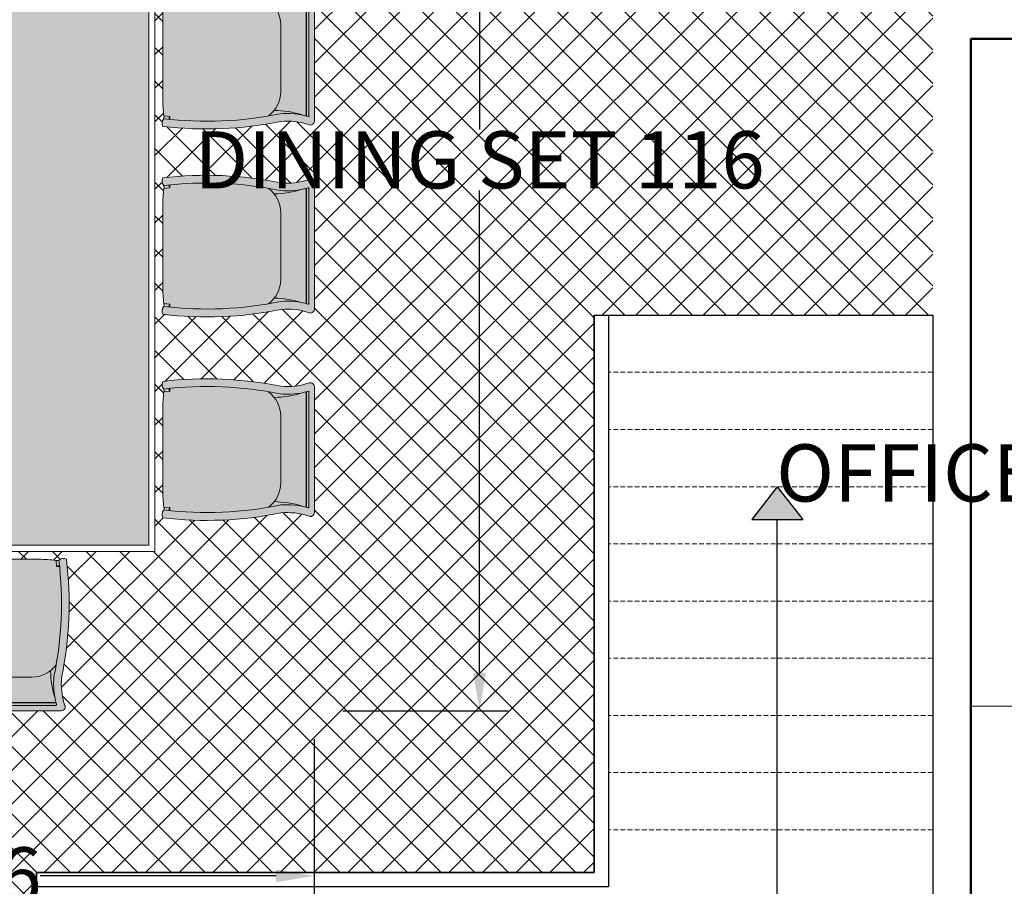
# Model space of a CAD drawing. Units: inches. Extents: x -466983 to 1020, y 324 to 318697.
# Tile 30 of 97: x 714 to 817, y 736 to 827. Entities that reach past the tile are written whole.
import ezdxf

# ---------------------------------------------------------------- set-up
doc = ezdxf.new("R2010")
doc.units = ezdxf.units.IN
doc.header["$MEASUREMENT"] = 0
doc.linetypes.add('DASHED', pattern=[0.75, 0.5, -0.25])
for name, color, linetype, lineweight in [('A-ANNO-DIMS', 2, 'Continuous', 18), ('A-FLOR-PATT', 252, 'Continuous', 13), ('A-FLOR-STRS', 30, 'Continuous', 25), ('A-FLOR-STRS-OVHD', 30, 'DASHED', 18), ('A-FURN', 8, 'Continuous', 18), ('A-WALL', 7, 'Continuous', 50)]:
    doc.layers.add(name, color=color, linetype=linetype, lineweight=lineweight)
doc.styles.get("Standard").update_dxf_attribs({"font": 'arial.ttf'})
doc.dimstyles.get("Standard").update_dxf_attribs({"dimtxt": 6, "dimasz": 4, "dimexe": 3, "dimexo": 3, "dimgap": 0.09, "dimtad": 0, "dimtih": 1, "dimtoh": 1, "dimdec": 1, "dimzin": 0, "dimdsep": 46, "dimlunit": 3, "dimtxsty": 'Standard', "dimcen": 0.09, "dimadec": 0, "dimazin": 0, "dimtfac": 1, "dimtdec": 1, "dimtofl": 0, "dimtmove": 0, "dimatfit": 3, "dimfxl": 1, "dimtolj": 1, "dimtzin": 0, "dimarcsym": 0})

# ---------------------------------------------------------------- blocks, each defined once
blk = doc.blocks.new('A$C51F1')
h = blk.add_hatch(color=256)
h.dxf.hatch_style = 1
h.paths.add_polyline_path([(0.4279, 0.4929), (0.026, 0.4929, 0.585109), (0.0153, 0.4737, -0.102523), (0.0249, 0.3863, 0.080461), (0.0093, 0.0091, 0.3023), (0.0338, 0.012, -0.012942), (0.0343, 0.0123, -0.080591), (0.05, 0.3835, 0.086627), (0.0435, 0.4661, -0.308377), (0.0433, 0.4665, -0.237278), (0.0433, 0.4671, 0.005839), (0.0418, 0.4726, -0.471786), (0.0436, 0.4758), (0.2273, 0.4758), (0.4111, 0.4758, -0.471786), (0.4129, 0.4726, 0.005839), (0.4114, 0.4671, -0.293853), (0.4112, 0.4664, 0.08699), (0.4047, 0.3835, -0.080655), (0.4203, 0.012, 0.301773), (0.4447, 0.0091, 0.080461), (0.4291, 0.3863, -0.102523), (0.4387, 0.4737, 0.587111)])
h.paths.add_polyline_path([(0.4107, 0.4676), (0.2273, 0.4676), (0.0439, 0.4676, 0.311255), (0.0433, 0.4671, -0.000568), (0.0434, 0.4666, -0.365297), (0.0439, 0.4668), (0.2273, 0.4668), (0.4107, 0.4668, -0.365297), (0.4113, 0.4666, -0.000568), (0.4114, 0.4671, 0.311255)], flags=17)
h = blk.add_hatch(color=256)
h.dxf.hatch_style = 1
h.paths.add_polyline_path([(0.4117, 0.3464, 0.23459), (0.3341, 0.3858), (0.2273, 0.3858), (0.1205, 0.3858, 0.165743), (0.061, 0.3649, 0.071703), (0.0463, 0.4542, -0.071168), (0.0502, 0.3861, 0.080361), (0.0343, 0.0123, -0.184513), (0.0429, 0.0127, 0.028193), (0.097, 0.0091), (0.227, 0.0091), (0.3571, 0.0091, 0.028193), (0.4111, 0.0127, -0.198751), (0.4203, 0.012, 0.072468)])
h.paths.add_polyline_path([(0.4084, 0.4542, -0.01323), (0.4113, 0.4666, 0.365297), (0.4107, 0.4668, 0.310553), (0.4107, 0.4676), (0.0439, 0.4676, 0.311255), (0.0433, 0.4671, -0.013798), (0.0463, 0.4542, -0.071703), (0.061, 0.3649, -0.165743), (0.1205, 0.3858), (0.2273, 0.3858), (0.3341, 0.3858, -0.165743), (0.3937, 0.3649, -0.071703)])
h.paths.add_polyline_path([(0.4047, 0.3835, -0.073923), (0.4084, 0.4542, 0.071703), (0.3937, 0.3649, -0.06627), (0.4117, 0.3464, 0.008137)], flags=17)
h.paths.add_polyline_path([(0.413, 0.473, 0.415817), (0.4111, 0.4758), (0.0436, 0.4758, 0.415817), (0.0416, 0.473, -0.006308), (0.0433, 0.4671, -0.311255), (0.0439, 0.4676), (0.4107, 0.4676, -0.336555), (0.4114, 0.4671, -0.006308)])
h = blk.add_hatch(color=256)
h.dxf.hatch_style = 1
h.paths.add_polyline_path([(0.4084, 0.4542, -0.01323), (0.4113, 0.4666, 0.365297), (0.4107, 0.4668), (0.2273, 0.4668), (0.0436, 0.4668, 0.193526), (0.0434, 0.4666, -0.01323), (0.0463, 0.4542, -0.071703), (0.061, 0.3649, -0.165743), (0.1205, 0.3858), (0.2273, 0.3858), (0.3341, 0.3858, -0.165743), (0.3937, 0.3649, -0.071703)])
at = {"color": 0}
for p, q in [((0.0436, 0.4758), (0.4111, 0.4758)), ((0.0439, 0.4676), (0.4107, 0.4676)), ((0.2273, 0.4668), (0.0439, 0.4668)), ((0.2273, 0.4668), (0.4107, 0.4668)), ((0.2273, 0.3858), (0.1205, 0.3858)), ((0.2273, 0.3858), (0.3341, 0.3858)), ((0.0417, 0.0321), (0.0321, 0.0321)), ((0.0417, 0.0321), (0.0326, 0.0278)), ((0.0435, 0.0127), (0.0417, 0.0321)), ((0.4112, 0.0127), (0.4129, 0.0321)), ((0.4129, 0.0321), (0.4225, 0.0321)), ((0.4129, 0.0321), (0.4221, 0.0278))]:
    blk.add_line(p, q, dxfattribs=at)
blk.add_lwpolyline([(0.4387, 0.4737, 0.102523), (0.4291, 0.3863, -0.080461), (0.4447, 0.0091, -0.3023), (0.4203, 0.012, 0.197932), (0.4111, 0.0127, -0.028193), (0.3571, 0.0091), (0.227, 0.0091), (0.097, 0.0091, -0.028193), (0.0429, 0.0127, 0.197932), (0.0338, 0.012, -0.3023), (0.0093, 0.0091, -0.080461), (0.0249, 0.3863, 0.102523), (0.0153, 0.4737, -0.587111), (0.0261, 0.4929), (0.4279, 0.4929, -0.587111)], format="xyb", close=True, dxfattribs=at)
for centre, radius, start, end in [((0.044, 0.4735), 0.00242, 100.345, 201.3742), ((-0.1898, 0.4063), 0.2409, 355.1793, 16.07), ((0.6445, 0.4063), 0.2409, 164.0374, 185.4487), ((0.4106, 0.4735), 0.00242, 338.6258, 79.655), ((0.0439, 0.4669), 0.000725, 87.3762, 197.5208), ((0.0438, 0.4664), 0.000433, 71.7715, 189.2202), ((-0.2563, 0.3584), 0.3173, 1.1591, 17.5641), ((0.7109, 0.3584), 0.3173, 162.4359, 178.8409), ((0.4107, 0.4669), 0.000725, 342.4792, 92.6238), ((0.4109, 0.4664), 0.000433, 350.7798, 108.2285), ((1.1976, 0.1501), 1.1714, 168.378, 186.769), ((0.1214, 0.2879), 0.0978, 90.5164, 143.1927), ((0.3332, 0.2879), 0.0978, 36.8073, 89.4836), ((-0.7314, 0.1497), 1.1599, 353.1854, 11.6291), ((0.0397, 0.0013), 0.012, 71.7536, 116.5375), ((0.4149, 0.0013), 0.012, 63.4625, 108.2464)]:
    blk.add_arc(centre, radius, start, end, dxfattribs=at)
blk = doc.blocks.new('Dining Table 1')
h = blk.add_hatch(color=256)
h.dxf.hatch_style = 1
h.set_gradient(color1=(0, 107, 0), color2=(254, 234, 185), name='INVSPHERICAL')
h.paths.add_polyline_path([(1939.98, 1142.68), (1908.44, 1142.68), (1908.44, 1061.84), (1939.98, 1061.84)])
at = {"ltscale": 0.5}
for points in [[(1907.78, 1143.33), (1907.78, 1061.19), (1940.64, 1061.19), (1940.64, 1143.33)], [(1908.44, 1142.68), (1908.44, 1061.84), (1939.98, 1061.84), (1939.98, 1142.68)]]:
    blk.add_lwpolyline(points, close=True, dxfattribs=at)
at = {"ltscale": 0.5, "xscale": 32.85880592291654, "yscale": 32.85880592291654, "zscale": 32.85880592291654}
blk.add_blockref('A$C51F1', (1916.75, 1143.86), dxfattribs=at)
at = {"ltscale": 0.5, "yscale": 32.85880592291654, "zscale": 32.85880592291654}
for p, xscale, rotation in [((1907.26, 1140.11), -32.85880592291654, 90), ((1941.16, 1140.11), 32.85880592291654, 270), ((1907.26, 1120.4), -32.85880592291654, 90), ((1941.16, 1120.4), 32.85880592291654, 270), ((1907.26, 1085.76), 32.85880592291654, 89.99999999999999), ((1941.16, 1085.76), -32.85880592291654, 270), ((1907.26, 1064.41), 32.85880592291654, 89.99999999999999), ((1941.16, 1064.41), -32.85880592291654, 270), ((1916.75, 1060.66), -32.85880592291654, 180)]:
    blk.add_blockref('A$C51F1', p, dxfattribs=dict(at, xscale=xscale, rotation=rotation))
blk = doc.blocks.new('*D99')
at = {"layer": 'A-ANNO-DIMS', "color": 0, "lineweight": -2, "transparency": 16777216}
for p, q in [((833.84, 822.68), (820.85, 822.68)), ((823.85, 818.68), (823.85, 782.57)), ((823.85, 740.08), (823.85, 776.18)), ((833.84, 736.08), (820.85, 736.08))]:
    blk.add_line(p, q, dxfattribs=at)
at = {"layer": 'A-ANNO-DIMS', "color": 0, "transparency": 16777216}
for points in [[(823.18, 818.68), (824.52, 818.68), (823.85, 822.68)], [(823.18, 740.08), (824.52, 740.08), (823.85, 736.08)]]:
    blk.add_solid(points, dxfattribs=at)
at = {"layer": 'Defpoints', "color": 0, "transparency": 16777216}
for p in [(823.85, 822.68), (836.84, 822.68), (836.84, 736.08)]:
    blk.add_point(p, dxfattribs=at)
at = {"layer": 'A-ANNO-DIMS', "color": 0, "transparency": 16777216, "insert": (823.85, 779.38), "char_height": 6, "attachment_point": 5}
blk.add_mtext('\\A1;OFFICE DESK 87', dxfattribs=at)
blk = doc.blocks.new('*D111')
at = {"layer": 'A-ANNO-DIMS', "color": 0, "lineweight": -2, "transparency": 16777216}
for p, q in [((747.94, 870.02), (765.28, 870.02)), ((762.28, 866.02), (762.28, 815.42)), ((762.28, 758.43), (762.28, 809.03)), ((747.94, 754.43), (765.28, 754.43))]:
    blk.add_line(p, q, dxfattribs=at)
at = {"layer": 'A-ANNO-DIMS', "color": 0, "transparency": 16777216}
for points in [[(761.61, 866.02), (762.95, 866.02), (762.28, 870.02)], [(761.61, 758.43), (762.95, 758.43), (762.28, 754.43)]]:
    blk.add_solid(points, dxfattribs=at)
at = {"layer": 'Defpoints', "color": 0, "transparency": 16777216}
for p in [(744.94, 870.02), (762.28, 870.02), (744.94, 754.43)]:
    blk.add_point(p, dxfattribs=at)
at = {"layer": 'A-ANNO-DIMS', "color": 0, "transparency": 16777216, "insert": (762.28, 812.23), "char_height": 6, "attachment_point": 5}
blk.add_mtext('\\A1;DINING SET 116', dxfattribs=at)
blk = doc.blocks.new('*D112')
at = {"layer": 'A-ANNO-DIMS', "color": 0, "lineweight": -2, "transparency": 16777216}
for p, q in [((678.65, 751.43), (678.65, 734.1)), ((744.94, 751.43), (744.94, 734.1)), ((682.65, 737.1), (707.39, 737.1)), ((740.94, 737.1), (716.2, 737.1))]:
    blk.add_line(p, q, dxfattribs=at)
at = {"layer": 'A-ANNO-DIMS', "color": 0, "transparency": 16777216}
for points in [[(682.65, 737.76), (682.65, 736.43), (678.65, 737.1)], [(740.94, 737.76), (740.94, 736.43), (744.94, 737.1)]]:
    blk.add_solid(points, dxfattribs=at)
at = {"layer": 'Defpoints', "color": 0, "transparency": 16777216}
for p in [(678.65, 754.43), (744.94, 754.43), (744.94, 737.1)]:
    blk.add_point(p, dxfattribs=at)
at = {"layer": 'A-ANNO-DIMS', "color": 0, "transparency": 16777216, "insert": (711.79, 737.1), "char_height": 6, "attachment_point": 5}
blk.add_mtext('\\A1;66', dxfattribs=at)

msp = doc.modelspace()

# ---------------------------------------------------------------- hatches: boundary and pattern name
at = {"layer": 'A-FLOR-PATT', "transparency": 33554572}
h = msp.add_hatch(dxfattribs=at)
h.set_pattern_fill('ANSI37', color=256, scale=30)
h.set_pattern_definition([(45, (-1212.4137, -290.035), (-2.6516504, 2.6516504), []), (135, (-1212.4137, -290.035), (-2.6516504, -2.6516504), [])])
h.paths.add_polyline_path([(901.81, 1075.94), (900.61, 1075.94), (900.61, 1065.39), (899.39, 1065.39), (898.09, 1065.39), (892.84, 1058.71, -0.258377), (892.19, 1058.35), (879.98, 1058.35, -0.20177), (879.44, 1058.58), (874.08, 1065.39), (872.78, 1065.39), (871.56, 1065.39), (871.56, 1075.94), (813.81, 1075.94), (813.81, 1044.79), (832.39, 1044.79, -0.394795), (848.66, 1028.54), (848.66, 1009.94), (901.81, 1009.94), (901.81, 1015.94), (901.31, 1015.94), (871.31, 1015.94), (871.31, 1017.25), (871.33, 1017.25, -0.401453), (901.31, 1045.94), (901.81, 1045.94)])
edge = h.paths.add_edge_path(flags=16)
edge.add_line((847.77, 1068.95), (847.77, 1073.71))
edge.add_arc((849.23, 1073.71), 1.45, 90, 180, ccw=False)
edge.add_line((849.23, 1075.16), (864.49, 1075.16))
edge.add_arc((864.49, 1073.71), 1.45, 0, 90, ccw=False)
edge.add_line((865.95, 1073.71), (865.95, 1069))
edge.add_arc((832.64, 1068.98), 33.3, -20.6123, 0.0472, ccw=False)
edge.add_ellipse((856.86, 1058.48), major_axis=(0, 10.21), ratio=0.685919, start_angle=100.0088, end_angle=259.9912, ccw=False)
edge.add_arc((881.07, 1068.98), 33.3, 180.0472, 200.6123, ccw=False)
h.paths.add_polyline_path([(853.15, 1066.48), (853.15, 1066.45), (853.15, 1066.45, 0.433107), (852.92, 1066.68), (852.92, 1066.45), (853.15, 1066.45), (853.15, 1066.48), (853.09, 1066.61, 0.697939), (852.7, 1066.45), (852.7, 1066.45), (852.7, 1066.48), (852.92, 1067), (852.92, 1066.68, -0.396254)], flags=0)
h.paths.add_polyline_path([(861.02, 1066.48), (861.02, 1066.45), (861.02, 1066.45, 0.416404), (860.8, 1066.68), (860.8, 1066.45), (861.02, 1066.45), (861.02, 1066.48), (860.97, 1066.61, 0.713344), (860.57, 1066.45), (860.57, 1066.45), (860.57, 1066.48), (860.8, 1067), (860.8, 1066.68, -0.379973)], flags=0)
edge = h.paths.add_edge_path(flags=0)
edge.add_spline(control_points=[(861.13, 1065.79), (861.47, 1065.25), (861.61, 1065.02), (861.98, 1064.37), (862.19, 1063.94), (862.56, 1063.04), (862.72, 1062.56), (862.99, 1061.58), (863.09, 1061.07), (863.25, 1060.03), (863.29, 1059.5), (863.33, 1058.44), (863.32, 1057.91), (863.24, 1056.85), (863.17, 1056.33), (862.97, 1055.31), (862.84, 1054.81), (862.54, 1053.85), (862.36, 1053.39), (861.95, 1052.52), (861.73, 1052.12), (861.23, 1051.36), (860.97, 1051.02), (860.4, 1050.39), (860.11, 1050.12), (859.49, 1049.65), (859.18, 1049.45), (858.53, 1049.13), (858.2, 1049.01), (857.53, 1048.85), (857.2, 1048.81), (856.52, 1048.81), (856.19, 1048.85), (855.52, 1049.01), (855.19, 1049.13), (854.54, 1049.45), (854.23, 1049.64), (853.61, 1050.12), (853.32, 1050.39), (852.75, 1051.01), (852.49, 1051.36), (852, 1052.11), (851.77, 1052.52), (851.36, 1053.39), (851.18, 1053.85), (850.88, 1054.81), (850.75, 1055.31), (850.55, 1056.33), (850.48, 1056.85), (850.4, 1057.9), (850.39, 1058.44), (850.43, 1059.5), (850.47, 1060.03), (850.63, 1061.07), (850.73, 1061.58), (851, 1062.56), (851.16, 1063.04), (851.53, 1063.94), (851.73, 1064.37), (852.11, 1065.02), (852.25, 1065.25), (852.61, 1065.73)], knot_values=[3.915332, 3.915332, 3.915332, 3.915332, 4.013468, 4.013468, 4.175532, 4.175532, 4.337596, 4.337596, 4.49966, 4.49966, 4.661724, 4.661724, 4.823788, 4.823788, 4.985852, 4.985852, 5.147916, 5.147916, 5.30998, 5.30998, 5.472044, 5.472044, 5.634109, 5.634109, 5.796173, 5.796173, 5.958237, 5.958237, 6.120301, 6.120301, 6.282365, 6.282365, 6.444429, 6.444429, 6.606493, 6.606493, 6.768557, 6.768557, 6.930621, 6.930621, 7.092685, 7.092685, 7.254749, 7.254749, 7.416813, 7.416813, 7.578878, 7.578878, 7.740942, 7.740942, 7.903006, 7.903006, 8.06507, 8.06507, 8.227134, 8.227134, 8.389198, 8.389198, 8.551262, 8.551262, 8.65037, 8.65037, 8.65037, 8.65037], degree=3, periodic=0)
edge.add_line((852.64, 1065.79), (861.13, 1065.79))
edge = h.paths.add_edge_path(flags=0)
edge.add_ellipse((856.85, 1057.74), major_axis=(0, 7.79), ratio=0.687861, start_angle=0, end_angle=360)
h.paths.add_polyline_path([(848.86, 1069.39), (848.86, 1073.96, -0.414214), (849.95, 1075.05), (863.77, 1075.05, -0.414214), (864.86, 1073.96), (864.86, 1069.39, -0.388936), (864.52, 1069.03, -0.043561), (849.2, 1069.03, -0.388936)], flags=0)
h.paths.add_polyline_path([(853.1, 1068.11, -1), (852.68, 1068.11, -1)], flags=0)
edge = h.paths.add_edge_path(flags=0)
edge.add_ellipse((856.86, 1057.34), major_axis=(0, 2.21), ratio=0.657164, start_angle=0, end_angle=360)
h.paths.add_polyline_path([(861.04, 1068.11, -1), (860.62, 1068.11, -1)], flags=0)
edge = h.paths.add_edge_path()
edge.add_line((573.95, 1057.34), (573.95, 1075.94))
edge.add_line((573.95, 1075.94), (558.73, 1075.94))
edge.add_line((558.73, 1075.94), (558.73, 1065.39))
edge.add_line((558.73, 1065.39), (557.51, 1065.39))
edge.add_line((557.51, 1065.39), (556.21, 1065.39))
edge.add_line((556.21, 1065.39), (550.95, 1058.71))
edge.add_arc((550.3, 1059.12), 0.765, 270, 327.9483, ccw=False)
edge.add_line((550.3, 1058.35), (538.1, 1058.35))
edge.add_arc((538.1, 1059.12), 0.765, 224.3704, 270, ccw=False)
edge.add_line((537.55, 1058.58), (532.2, 1065.39))
edge.add_line((532.2, 1065.39), (530.9, 1065.39))
edge.add_line((530.9, 1065.39), (529.67, 1065.39))
edge.add_line((529.67, 1065.39), (529.67, 1075.94))
edge.add_line((529.67, 1075.94), (520.81, 1075.94))
edge.add_line((520.81, 1075.94), (520.81, 1045.94))
edge.add_line((520.81, 1045.94), (521.31, 1045.94))
edge.add_arc((521.31, 1015.94), 30, 2.5075, 90, ccw=False)
edge.add_line((551.28, 1017.25), (551.31, 1017.25))
edge.add_line((551.31, 1017.25), (551.31, 1015.94))
edge.add_line((551.31, 1015.94), (520.81, 1015.94))
edge.add_line((520.81, 1015.94), (520.81, 1009.94))
edge.add_line((520.81, 1009.94), (559.19, 1010.4))
edge.add_arc((559.19, 1011.86), 1.45, 180, 270, ccw=False)
edge.add_line((557.74, 1011.86), (557.74, 1016.56))
edge.add_arc((591.04, 1016.59), 33.3, 159.3877, 180.0472, ccw=False)
edge.add_ellipse((566.82, 1027.08), major_axis=(0, 10.21), ratio=0.685919, start_angle=280.0088, end_angle=439.9912, ccw=False)
edge.add_arc((542.61, 1016.59), 33.3, 0.0472, 20.6123, ccw=False)
edge.add_line((575.91, 1016.62), (575.91, 1011.86))
edge.add_arc((574.46, 1011.86), 1.45, -90, 0, ccw=False)
edge.add_line((574.46, 1010.4), (608.81, 1009.94))
edge.add_line((608.81, 1009.94), (608.81, 1041.09))
edge.add_line((608.81, 1041.09), (590.22, 1041.09))
edge.add_arc((590.78, 1057.91), 16.83, 181.9277, 268.1032, ccw=False)
edge = h.paths.add_edge_path()
edge.add_ellipse((494.24, 583.62), major_axis=(0, 10.21), ratio=0.685919, start_angle=280.0088, end_angle=439.9912, ccw=False)
edge.add_arc((470.03, 573.12), 33.3, 0.0472, 20.6123, ccw=False)
edge.add_line((503.33, 573.15), (503.33, 568.39))
edge.add_arc((501.88, 568.39), 1.45, -90, 0, ccw=False)
edge.add_line((501.88, 566.94), (539.81, 566.94))
edge.add_line((539.81, 566.94), (539.81, 572.94))
edge.add_line((539.81, 572.94), (539.31, 572.94))
edge.add_line((539.31, 572.94), (509.31, 572.94))
edge.add_line((509.31, 572.94), (509.31, 574.25))
edge.add_line((509.31, 574.25), (509.33, 574.25))
edge.add_arc((539.31, 572.94), 30, 90, 177.4925, ccw=False)
edge.add_line((539.31, 602.94), (539.81, 602.94))
edge.add_line((539.81, 602.94), (539.81, 626.94))
edge.add_line((539.81, 626.94), (531.77, 626.94))
edge.add_line((531.77, 626.94), (531.77, 616.39))
edge.add_line((531.77, 616.39), (530.55, 616.39))
edge.add_line((530.55, 616.39), (529.25, 616.39))
edge.add_line((529.25, 616.39), (523.71, 609.35))
edge.add_line((523.71, 609.35), (510.78, 609.35))
edge.add_line((510.78, 609.35), (505.24, 616.39))
edge.add_line((505.24, 616.39), (503.94, 616.39))
edge.add_line((503.94, 616.39), (502.72, 616.39))
edge.add_line((502.72, 616.39), (502.72, 626.94))
edge.add_line((502.72, 626.94), (481.7, 626.94))
edge.add_line((481.7, 626.94), (481.7, 611))
edge.add_arc((467.27, 611.47), 14.44, 271.9277, 358.1032, ccw=False)
edge.add_line((467.76, 597.05), (451.81, 597.05))
edge.add_line((451.81, 597.05), (451.81, 584.4))
edge.add_line((451.81, 584.4), (451.81, 566.94))
edge.add_line((451.81, 566.94), (486.61, 566.94))
edge.add_arc((486.61, 568.39), 1.45, 180, 270, ccw=False)
edge.add_line((485.16, 568.39), (485.16, 573.1))
edge.add_arc((518.46, 573.12), 33.3, 159.3877, 180.0472, ccw=False)
h.paths.add_polyline_path([(836.26, 1020.73), (879.89, 1020.73), (879.89, 1039.39), (836.26, 1039.39)], flags=25)
h.paths.add_polyline_path([(549.99, 1036.75), (593.61, 1036.75), (593.61, 1055.41), (549.99, 1055.41)], flags=24)
h.paths.add_polyline_path([(475.12, 595.6), (518.75, 595.6), (518.75, 614.25), (475.12, 614.25)], flags=24)
h = msp.add_hatch(dxfattribs=at)
h.set_pattern_fill('ANSI37', color=256, scale=20)
h.set_pattern_definition([(45, (-1212.4137, -290.035), (-1.767767, 1.767767), []), (135, (-1212.4137, -290.035), (-1.767767, -1.767767), [])])
h.paths.add_polyline_path([(809.81, 870.94), (809.81, 888.15), (807, 888.15), (802.66, 888.15), (789.38, 888.15), (786.28, 888.15, -0.414214), (785.5, 888.94), (785.5, 900.2), (785.5, 908.47, -0.414214), (786.81, 909.78, -0.414214), (785.5, 911.09), (785.5, 929.1, -0.414214), (786.81, 930.41, -0.414214), (785.5, 931.72), (785.5, 931.9, -0.414214), (784.19, 930.59), (766.72, 930.59, -0.412359), (765.41, 931.9, -0.413741), (764.11, 930.58), (744.58, 930.42, -0.416556), (743.79, 931.21), (743.79, 933.52), (742.22, 933.52), (742.22, 952.02, -0.001344), (743.79, 952.2), (743.79, 953.94), (678.59, 953.94), (678.59, 951.13), (678.59, 946.79), (678.59, 933.52), (678.59, 930.42, -0.414214), (677.81, 929.63), (666.55, 929.63), (658.27, 929.63, -0.414214), (656.96, 930.94, -0.414214), (655.66, 929.63), (637.64, 929.63, -0.414214), (636.33, 930.94, -0.414214), (635.02, 929.63), (634.84, 929.63, -0.414214), (636.15, 928.32), (636.15, 910.85, -0.412359), (634.85, 909.55, -0.413741), (636.17, 908.25), (636.32, 888.71, -0.416556), (635.54, 887.92), (633.23, 887.92), (633.23, 886.35), (614.72, 886.35, -0.001344), (614.54, 887.92), (612.81, 887.92), (612.81, 834.94), (612.81, 752.94), (612.81, 748.94), (612.81, 697.94), (654.81, 697.94), (654.81, 701.94), (715.81, 701.94), (715.81, 737.44), (774.29, 737.44), (774.29, 795.94), (809.81, 795.94)])
h.paths.add_polyline_path([(679.28, 849.58, 0.102523), (682.15, 849.26, -0.080461), (694.54, 849.77, -0.283899), (694.48, 849.01, 0.136605), (694.41, 848.81, -0.030441), (694.54, 846.89), (694.54, 842.62), (694.54, 838.35, -0.028219), (694.42, 836.57), (694.43, 836.57, 0.196187), (694.45, 836.27, -0.302897), (694.54, 835.47, -0.080461), (682.15, 835.98, 0.102523), (679.28, 835.66, -0.58611), (678.65, 836.02), (678.65, 849.22, -0.58611)], flags=16)
h.paths.add_polyline_path([(679.52, 848.65, 0.699597), (679.48, 848.63, 1.20716), (679.19, 848.74, 0.010621)], flags=0)
h.paths.add_polyline_path([(679.49, 836.56, -0.013798), (679.92, 836.66, -0.071703), (682.85, 837.14, -0.165743), (682.17, 839.1), (682.17, 842.61), (682.17, 846.06, -0.240616), (683.47, 848.68, -0.068263), (693.93, 849.01), (693.79, 848.71), (693.79, 849.02, 0.067332), (683.47, 848.68, 0.240616), (682.17, 846.06), (682.17, 842.61), (682.17, 839.1, 0.23459), (683.46, 836.55, 0.068093), (693.79, 836.2), (693.79, 836.51), (693.93, 836.21, -0.077215), (682.24, 836.78, 0.086627), (679.53, 836.57, -0.628402), (679.5, 836.57), (679.5, 836.61, 0.910458)], flags=0)
h.paths.add_polyline_path([(679.48, 848.64), (679.21, 848.65), (679.21, 836.57, 0.913566), (679.36, 836.59), (679.48, 836.58)], flags=0)
h.paths.add_polyline_path([(679.28, 829.86, 0.102523), (682.15, 829.55, -0.080461), (694.54, 830.06, -0.283899), (694.48, 829.29, 0.136605), (694.41, 829.1, -0.030441), (694.54, 827.18), (694.54, 822.9), (694.54, 818.63, -0.028219), (694.42, 816.85), (694.43, 816.85, 0.196187), (694.45, 816.56, -0.302897), (694.54, 815.75, -0.080461), (682.15, 816.26, 0.102523), (679.28, 815.95, -0.58611), (678.65, 816.3), (678.65, 829.51, -0.58611)], flags=16)
h.paths.add_polyline_path([(679.52, 828.94, 0.699597), (679.48, 828.92, 1.20716), (679.19, 829.03, 0.010621)], flags=0)
h.paths.add_polyline_path([(679.49, 816.85, -0.013798), (679.92, 816.94, -0.071703), (682.85, 817.43, -0.165743), (682.17, 819.39), (682.17, 822.89), (682.17, 826.34, -0.240616), (683.47, 828.96, -0.068263), (693.93, 829.29), (693.79, 828.99), (693.79, 829.31, 0.067332), (683.47, 828.96, 0.240616), (682.17, 826.34), (682.17, 822.89), (682.17, 819.39, 0.23459), (683.46, 816.84, 0.068093), (693.79, 816.48), (693.79, 816.8), (693.93, 816.49, -0.077215), (682.24, 817.07, 0.086627), (679.53, 816.85, -0.628402), (679.5, 816.86), (679.5, 816.89, 0.910458)], flags=0)
h.paths.add_polyline_path([(679.48, 828.92), (679.21, 828.93), (679.21, 816.86, 0.913566), (679.36, 816.87), (679.48, 816.87)], flags=0)
h.paths.add_polyline_path([(679.28, 810.15, 0.102523), (682.15, 809.83, -0.080461), (694.54, 810.34, -0.3023), (694.45, 809.54, 0.10023), (694.41, 809.39, -0.03057), (694.54, 807.46), (694.54, 803.19), (694.54, 798.92, -0.03057), (694.41, 796.99, 0.10023), (694.45, 796.84, -0.3023), (694.54, 796.04, -0.080461), (682.15, 796.55, 0.102523), (679.28, 796.23, -0.58611), (678.65, 796.59), (678.65, 809.79, -0.58611)], flags=16)
h.paths.add_polyline_path([(679.52, 809.24, 0.699597), (679.48, 809.22, 1.20716), (679.19, 809.33, 0.010621)], flags=0)
h.paths.add_polyline_path([(679.49, 797.15, -0.013798), (679.92, 797.25, -0.071703), (682.85, 797.73, -0.165743), (682.17, 799.69), (682.17, 803.2), (682.17, 806.65, -0.239349), (683.46, 809.26, -0.072465), (694.45, 809.54, 0.197932), (694.43, 809.24), (693.79, 809.3), (693.79, 809.61, 0.068093), (683.46, 809.26, 0.239349), (682.17, 806.65), (682.17, 803.2), (682.17, 799.69, 0.235854), (683.47, 797.13, 0.067332), (693.79, 796.79), (693.79, 797.1), (694.43, 797.16, 0.197932), (694.45, 796.86, -0.080419), (682.16, 797.38, 0.083867), (679.53, 797.16, -0.628402), (679.5, 797.16), (679.5, 797.2, 0.910458)], flags=0)
h.paths.add_polyline_path([(679.21, 809.24), (679.21, 797.16, 0.913566), (679.36, 797.18), (679.48, 797.17), (679.48, 809.23)], flags=0)
h.paths.add_polyline_path([(695.36, 853.3), (728.22, 853.3), (728.22, 771.15), (695.36, 771.15)], flags=16)
h.paths.add_polyline_path([(696.02, 852.64), (727.57, 852.64), (727.57, 771.81), (696.02, 771.81)], flags=0)
h.paths.add_polyline_path([(679.28, 788.79, 0.102523), (682.15, 788.47, -0.080461), (694.54, 788.98, -0.3023), (694.45, 788.18, 0.10023), (694.41, 788.03, -0.03057), (694.54, 786.1), (694.54, 781.83), (694.54, 777.56, -0.03057), (694.41, 775.63, 0.10023), (694.45, 775.48, -0.3023), (694.54, 774.68, -0.080461), (682.15, 775.19, 0.102523), (679.28, 774.88, -0.58611), (678.65, 775.23), (678.65, 788.43, -0.58611)], flags=16)
h.paths.add_polyline_path([(679.52, 787.88, 0.699597), (679.48, 787.87, 1.20716), (679.19, 787.97, 0.010621)], flags=0)
h.paths.add_polyline_path([(679.49, 775.79, -0.013798), (679.92, 775.89, -0.071703), (682.85, 776.38, -0.165743), (682.17, 778.33), (682.17, 781.84), (682.17, 785.29, -0.239349), (683.46, 787.9, -0.072465), (694.45, 788.18, 0.197932), (694.43, 787.88), (693.79, 787.94), (693.79, 788.26, 0.068093), (683.46, 787.9, 0.239349), (682.17, 785.29), (682.17, 781.84), (682.17, 778.33, 0.235854), (683.47, 775.77, 0.067332), (693.79, 775.43), (693.79, 775.74), (694.43, 775.8, 0.197932), (694.45, 775.5, -0.080419), (682.16, 776.02, 0.083867), (679.53, 775.8, -0.628402), (679.5, 775.81), (679.5, 775.84, 0.910458)], flags=0)
h.paths.add_polyline_path([(679.21, 787.88), (679.21, 775.8, 0.913566), (679.36, 775.82), (679.48, 775.81), (679.48, 787.87)], flags=0)
h.paths.add_polyline_path([(704.64, 854.12, -0.080461), (705.15, 866.52, 0.102523), (704.84, 869.39, -0.58611), (705.19, 870.02), (718.4, 870.02, -0.58611), (718.75, 869.39, 0.102523), (718.43, 866.52, -0.080461), (718.95, 854.12, -0.3023), (718.14, 854.22, 0.10023), (717.99, 854.26, -0.03057), (716.07, 854.12), (711.79, 854.12), (707.52, 854.12, -0.03057), (705.6, 854.26, 0.10023), (705.44, 854.22, -0.3023)], flags=16)
h.paths.add_polyline_path([(717.85, 869.15, 0.699597), (717.83, 869.19, 1.20716), (717.94, 869.47, 0.010621)], flags=0)
h.paths.add_polyline_path([(705.46, 854.22, -0.080419), (705.98, 866.51, 0.083867), (705.76, 869.13, -0.628402), (705.77, 869.16), (705.8, 869.16, 0.910458), (705.76, 869.17, -0.013798), (705.85, 868.75, -0.071703), (706.34, 865.81, -0.165743), (708.3, 866.5), (711.8, 866.5), (715.25, 866.5, -0.239349), (717.86, 865.2, -0.072465), (718.15, 854.22, 0.197932), (717.85, 854.24), (717.9, 854.88), (718.22, 854.88, 0.068093), (717.86, 865.2, 0.239349), (715.25, 866.5), (711.8, 866.5), (708.3, 866.5, 0.235854), (705.74, 865.19, 0.067332), (705.39, 854.88), (705.71, 854.88), (705.76, 854.24, 0.197932)], flags=16)
h.paths.add_polyline_path([(705.77, 869.46, 0.913566), (705.78, 869.3), (705.78, 869.19), (717.83, 869.19), (717.84, 869.46)], flags=0)
h.paths.add_polyline_path([(729.04, 842.62), (729.04, 846.89, -0.03057), (729.18, 848.82, 0.10023), (729.14, 848.97, -0.3023), (729.04, 849.77, -0.080461), (741.44, 849.26, 0.102523), (744.31, 849.58, -0.58611), (744.94, 849.22), (744.94, 836.02, -0.58611), (744.31, 835.66, 0.102523), (741.44, 835.98, -0.080461), (729.04, 835.47, -0.3023), (729.14, 836.27, 0.10023), (729.18, 836.42, -0.03057), (729.04, 838.35)], flags=16)
h.paths.add_polyline_path([(744.11, 836.58, 1.20716), (744.39, 836.48, 0.010621), (744.07, 836.57, 0.699597)], flags=0)
h.paths.add_polyline_path([(729.14, 836.27, 0.197932), (729.16, 836.57), (729.8, 836.51), (729.8, 836.2, 0.068093), (740.13, 836.55, 0.239349), (741.42, 839.16), (741.42, 842.61), (741.42, 846.12, 0.235854), (740.11, 848.68, 0.067332), (729.8, 849.02), (729.8, 848.71), (729.16, 848.65, 0.197932), (729.14, 848.95, -0.080419), (741.43, 848.43, 0.083867), (744.06, 848.65, -0.628402), (744.08, 848.65), (744.08, 848.61, 0.910458), (744.1, 848.66, -0.013798), (743.67, 848.56, -0.071703), (740.73, 848.08, -0.165743), (741.42, 846.12), (741.42, 842.61), (741.42, 839.16, -0.239349), (740.13, 836.55, -0.072465)], flags=0)
h.paths.add_polyline_path([(729.04, 830.06, -0.080461), (741.44, 829.55, 0.102523), (744.31, 829.86, -0.58611), (744.94, 829.51), (744.94, 816.3, -0.58611), (744.31, 815.95, 0.102523), (741.44, 816.26, -0.080461), (729.04, 815.75, -0.3023), (729.14, 816.55, 0.10023), (729.18, 816.71, -0.03057), (729.04, 818.63), (729.04, 822.9), (729.04, 827.18, -0.03057), (729.18, 829.1, 0.10023), (729.14, 829.25, -0.3023)], flags=16)
h.paths.add_polyline_path([(744.11, 816.87, 1.20716), (744.39, 816.76, 0.010621), (744.07, 816.85, 0.699597)], flags=0)
h.paths.add_polyline_path([(729.14, 829.24, -0.080419), (741.43, 828.71, 0.083867), (744.06, 828.93, -0.628402), (744.08, 828.93), (744.08, 828.9, 0.910458), (744.1, 828.94, -0.013798), (743.67, 828.84, -0.071703), (740.73, 828.36, -0.165743), (741.42, 826.4), (741.42, 822.89), (741.42, 819.44, -0.239349), (740.13, 816.84, -0.072465), (729.14, 816.55, 0.197932), (729.16, 816.85), (729.8, 816.8), (729.8, 816.48, 0.068093), (740.13, 816.84, 0.239349), (741.42, 819.44), (741.42, 822.89), (741.42, 826.4, 0.235854), (740.11, 828.96, 0.067332), (729.8, 829.31), (729.8, 828.99), (729.16, 828.94, 0.197932)], flags=16)
h.paths.add_polyline_path([(729.04, 810.34, -0.080461), (741.44, 809.83, 0.102523), (744.31, 810.15, -0.58611), (744.94, 809.79), (744.94, 796.59, -0.58611), (744.31, 796.23, 0.102523), (741.44, 796.55, -0.080461), (729.04, 796.04, -0.283899), (729.11, 796.8, 0.136605), (729.18, 797, -0.030441), (729.04, 798.92), (729.04, 803.19), (729.04, 807.46, -0.028219), (729.16, 809.24), (729.16, 809.24, 0.196187), (729.14, 809.54, -0.302897)], flags=16)
h.paths.add_polyline_path([(744.11, 797.17, 1.20716), (744.39, 797.07, 0.010621), (744.07, 797.16, 0.699597)], flags=0)
h.paths.add_polyline_path([(741.35, 809.03, 0.086627), (744.06, 809.24, -0.628402), (744.08, 809.24), (744.08, 809.2, 0.910458), (744.1, 809.25, -0.013798), (743.67, 809.15, -0.071703), (740.73, 808.67, -0.165743), (741.42, 806.71), (741.42, 803.2), (741.42, 799.75, -0.240616), (740.11, 797.13, -0.068263), (729.66, 796.8), (729.8, 797.1), (729.8, 796.79, 0.067332), (740.11, 797.13, 0.240616), (741.42, 799.75), (741.42, 803.2), (741.42, 806.71, 0.23459), (740.13, 809.26, 0.068093), (729.8, 809.61), (729.8, 809.3), (729.66, 809.6, -0.077215)], flags=0)
h.paths.add_polyline_path([(704.64, 770.33, -0.283899), (705.41, 770.27, 0.136605), (705.6, 770.19, -0.030441), (707.52, 770.33), (711.79, 770.33), (716.07, 770.33, -0.028219), (717.85, 770.21), (717.85, 770.21, 0.196187), (718.14, 770.23, -0.302897), (718.95, 770.33, -0.080461), (718.43, 757.94, 0.102523), (718.75, 755.06, -0.58611), (718.4, 754.43), (705.19, 754.43, -0.58611), (704.84, 755.06, 0.102523), (705.15, 757.94, -0.080461)], flags=16)
h.paths.add_polyline_path([(705.76, 755.3, 0.699597), (705.78, 755.26, 1.20716), (705.67, 754.98, 0.010621)], flags=0)
h.paths.add_polyline_path([(705.41, 769.72), (705.71, 769.58), (705.39, 769.58, 0.067332), (705.74, 759.26, 0.240616), (708.35, 757.95), (711.8, 757.95), (715.31, 757.95, 0.23459), (717.86, 759.25, 0.068093), (718.22, 769.58), (717.9, 769.58), (718.2, 769.72, -0.077215), (717.63, 758.03, 0.086627), (717.84, 755.32, -0.628402), (717.84, 755.29), (717.81, 755.29, 0.910458), (717.85, 755.28, -0.013798), (717.75, 755.71, -0.071703), (717.27, 758.64, -0.165743), (715.31, 757.95), (711.8, 757.95), (708.35, 757.95, -0.240616), (705.74, 759.26, -0.068263)], flags=0)
h.paths.add_polyline_path([(729.04, 788.98, -0.080461), (741.44, 788.47, 0.102523), (744.31, 788.79, -0.58611), (744.94, 788.43), (744.94, 775.23, -0.58611), (744.31, 774.88, 0.102523), (741.44, 775.19, -0.080461), (729.04, 774.68, -0.283899), (729.11, 775.44, 0.136605), (729.18, 775.64, -0.030441), (729.04, 777.56), (729.04, 781.83), (729.04, 786.1, -0.028219), (729.16, 787.88), (729.16, 787.88, 0.196187), (729.14, 788.18, -0.302897)], flags=16)
h.paths.add_polyline_path([(744.11, 775.82, 1.20716), (744.39, 775.71, 0.010621), (744.07, 775.8, 0.699597)], flags=0)
h.paths.add_polyline_path([(741.35, 787.67, 0.086627), (744.06, 787.88, -0.628402), (744.08, 787.88), (744.08, 787.84, 0.910458), (744.1, 787.89, -0.013798), (743.67, 787.79, -0.071703), (740.73, 787.31, -0.165743), (741.42, 785.35), (741.42, 781.84), (741.42, 778.39, -0.240616), (740.11, 775.77, -0.068263), (729.66, 775.44), (729.8, 775.74), (729.8, 775.43, 0.067332), (740.11, 775.77, 0.240616), (741.42, 778.39), (741.42, 781.84), (741.42, 785.35, 0.23459), (740.13, 787.9, 0.068093), (729.8, 788.26), (729.8, 787.94), (729.66, 788.24, -0.077215)], flags=0)
h.paths.add_polyline_path([(744.11, 848.64), (744.11, 836.58), (744.38, 836.57), (744.38, 848.65, 0.913566), (744.22, 848.63)], flags=0)
h.paths.add_polyline_path([(744.22, 828.92), (744.11, 828.92), (744.11, 816.87), (744.38, 816.86), (744.38, 828.93, 0.913566)], flags=0)
h.paths.add_polyline_path([(717.83, 755.26), (705.78, 755.26), (705.77, 754.99), (717.84, 754.99, 0.913566), (717.83, 755.15)], flags=0)
h.paths.add_polyline_path([(744.22, 809.22), (744.11, 809.23), (744.11, 797.17), (744.38, 797.16), (744.38, 809.24, 0.913566)], flags=0)
h.paths.add_polyline_path([(744.11, 787.87), (744.11, 775.81), (744.38, 775.8), (744.38, 787.88, 0.913566), (744.22, 787.86)], flags=0)
h.paths.add_polyline_path([(678.88, 877.12), (737.61, 877.12), (737.61, 899.51), (678.88, 899.51)], flags=24)
at = {"layer": 'A-FLOR-STRS'}
h = msp.add_hatch(color=256, dxfattribs=at)
h.dxf.hatch_style = 1
h.paths.add_polyline_path([(793.49, 777.94), (790.82, 774.5), (796.17, 774.5)])

# ---------------------------------------------------------------- linework, layer by layer
for p, q in [((774.29, 795.94), (774.29, 737.44)), ((793.49, 777.94), (790.82, 774.5)), ((793.49, 777.94), (796.17, 774.5)), ((790.82, 774.5), (796.17, 774.5)), ((793.49, 716.06), (793.49, 774.5)), ((715.81, 737.44), (715.81, 701.94)), ((774.29, 737.44), (715.81, 737.44))]:
    msp.add_line(p, q, dxfattribs=at)
msp.add_lwpolyline([(774.29, 737.44), (774.29, 795.94), (809.81, 795.94), (809.81, 701.94), (715.81, 701.94), (715.81, 737.44)], close=True, dxfattribs=at)
msp.add_lwpolyline([(775.81, 795.94), (775.81, 735.94), (715.81, 735.94)], dxfattribs=at)
at = {"layer": 'A-FLOR-STRS-OVHD'}
for p, q in [((809.81, 795.94), (774.29, 795.94)), ((809.81, 789.94), (775.81, 789.94)), ((809.81, 783.94), (775.81, 783.94)), ((809.81, 777.94), (775.81, 777.94)), ((809.81, 771.94), (775.81, 771.94)), ((809.81, 765.94), (775.81, 765.94)), ((809.81, 759.94), (775.81, 759.94)), ((809.81, 753.94), (775.81, 753.94)), ((809.81, 747.94), (775.81, 747.94)), ((809.81, 741.94), (775.81, 741.94))]:
    msp.add_line(p, q, dxfattribs=at)
at = {"layer": 'A-FURN', "elevation": -0.02}
msp.add_lwpolyline([(836.84, 754.9), (813.81, 754.9), (813.81, 824.94), (836.92, 824.94), (836.92, 754.9)], dxfattribs=at)
at = {"layer": 'A-WALL'}
for p, q in [((982.81, 824.94), (813.81, 824.94)), ((813.81, 824.94), (813.81, 691.94))]:
    msp.add_line(p, q, dxfattribs=at)

# ---------------------------------------------------------------- block references
at = {"layer": 'A-FURN'}
msp.add_blockref('Dining Table 1', (-1212.41, -290.04), dxfattribs=at)

# ---------------------------------------------------------------- dimensions: what is measured, and where the dimension line sits
at = {"layer": 'A-ANNO-DIMS'}
for base, p1, p2, text, picture, middle in [((762.28, 870.02), (744.94, 754.43), (744.94, 870.02), 'DINING SET <>', '*D111', (762.28, 812.23)), ((823.85, 822.68), (836.84, 736.08), (836.84, 822.68), 'OFFICE DESK <>', '*D99', (823.85, 779.38))]:
    dim = msp.add_linear_dim(base=base, p1=p1, p2=p2, angle=90, text=text, dimstyle='Standard', override={"dimdec": 0, "dimlfac": 1, "dimrnd": 0, "dimzin": 0, "dimdsep": 46, "dimlunit": 2}, dxfattribs=at)
    dim.commit()
    dim.dimension.update_dxf_attribs({"geometry": picture, "text_midpoint": middle})
dim = msp.add_linear_dim(base=(744.94, 737.1), p1=(678.65, 754.43), p2=(744.94, 754.43), dimstyle='Standard', override={"dimdec": 0, "dimlfac": 1, "dimrnd": 0, "dimzin": 0, "dimdsep": 46, "dimlunit": 2}, dxfattribs=at)
dim.commit()
dim.dimension.update_dxf_attribs({"geometry": '*D112', "text_midpoint": (711.79, 737.1)})

doc.saveas('drawing.dxf')
